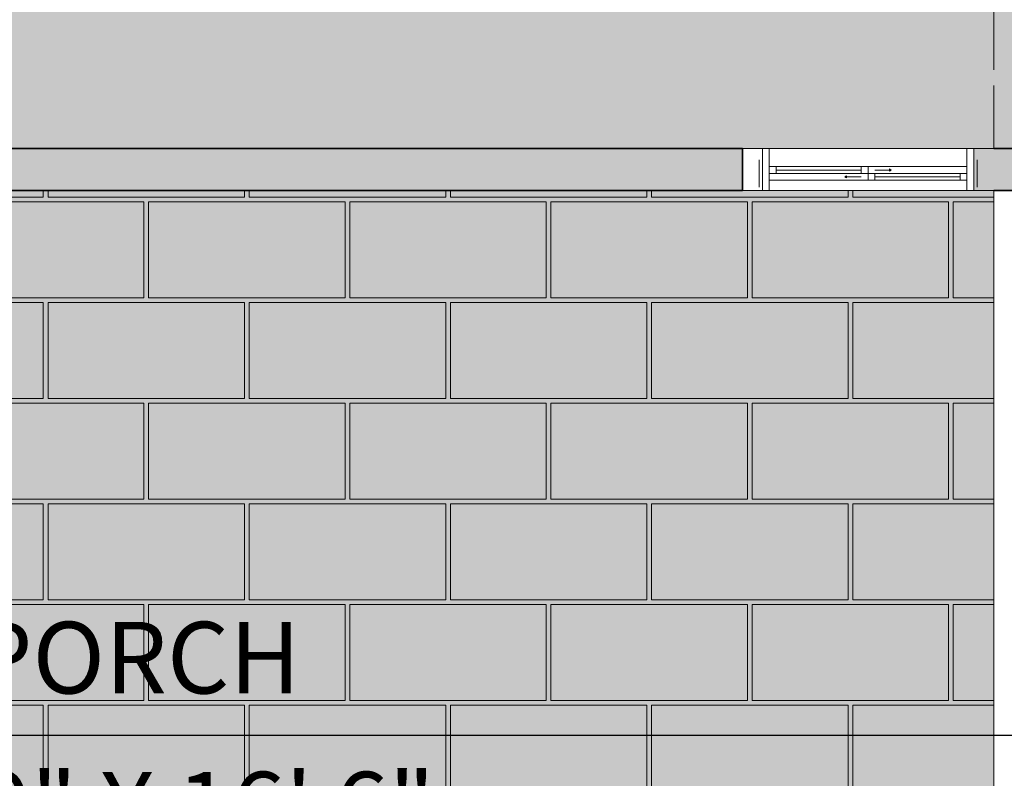
# Model space of a CAD drawing. Units: inches. Extents: x 1704 to 6393, y -157 to 1172.
# Tile 20 of 122: x 2087 to 2275, y 82 to 227. Entities that reach past the tile are written whole.
import ezdxf

# ---------------------------------------------------------------- set-up
doc = ezdxf.new("R2010")
doc.units = ezdxf.units.IN
doc.header["$MEASUREMENT"] = 0
doc.linetypes.add('ACAD_ISO02W100', pattern=[15, 12, -3])
for name, color, linetype, lineweight in [('A-ANNO-DIMS', 7, 'Continuous', 13), ('A-AREA-IDEN', 7, 'Continuous', 18), ('A-WALL-OVHD', 8, 'ACAD_ISO02W100', 13), ('A-WALL-PATT', 7, 'Continuous', 13), ('L-HRDS', 8, 'Continuous', 18), ('L-PVMT-PATT', 8, 'Continuous', 13), ('WALLS', 7, 'Continuous', 35), ('WINDOWS', 2, 'Continuous', 18)]:
    doc.layers.add(name, color=color, linetype=linetype, lineweight=lineweight)
doc.layers.add('A-FLOR-PATT', color=7, linetype='Continuous', lineweight=13, true_color=0xf2f2f2)
doc.layers.add('L-HRDS-PATT', color=9, linetype='Continuous', lineweight=13, true_color=0xc5c1ba)
doc.styles.get("Standard").update_dxf_attribs({"font": 'arial.ttf'})
doc.dimstyles.get("Standard").update_dxf_attribs({"dimtxt": 6, "dimasz": 2, "dimexe": 0.18, "dimexo": 0.0625, "dimgap": 0.09, "dimtad": 0, "dimtih": 1, "dimtoh": 1, "dimdec": 1, "dimzin": 0, "dimdsep": 46, "dimlunit": 3, "dimtxsty": 'Standard', "dimblk": 'ARCHTICK', "dimcen": 0.09, "dimadec": 0, "dimazin": 0, "dimtfac": 1, "dimtdec": 1, "dimtofl": 0, "dimtmove": 0, "dimatfit": 3, "dimfxl": 1, "dimtolj": 1, "dimtzin": 0, "dimarcsym": 0})

# ---------------------------------------------------------------- blocks, each defined once
blk = doc.blocks.new('WIN-SLIDER-48')
for p, q in [((3.83, 8), (0, 8)), ((5.13, 8), (42.87, 8)), ((44.17, 8), (48, 8)), ((3.18, 5.86), (3.18, 0.65)), ((44.82, 5.86), (44.82, 0.65)), ((6.43, 4.55), (22.7, 4.55)), ((6.43, 3.9), (22.7, 3.9)), ((24, 4.55), (42.87, 4.55)), ((25.3, 3.9), (28.1, 3.9)), ((24, 1.95), (5.13, 1.95)), ((6.43, 3.25), (22.7, 3.25)), ((22.7, 2.6), (19.9, 2.6)), ((25.3, 3.25), (41.56, 3.25)), ((25.3, 2.6), (41.56, 2.6)), ((25.3, 1.95), (41.56, 1.95)), ((3.83, 0), (0, 0)), ((5.13, 0), (42.87, 0)), ((44.17, 0), (48, 0))]:
    blk.add_line(p, q)
for points in [[(5.13, 0), (3.83, 0), (3.83, 8), (5.13, 8)], [(42.87, 0), (44.17, 0), (44.17, 8), (42.87, 8)], [(5.13, 3.25), (6.43, 3.25), (6.43, 4.55), (5.13, 4.55)], [(22.7, 3.25), (24, 3.25), (24, 4.55), (22.7, 4.55)], [(28.43, 3.9), (28.1, 4.1), (28.1, 3.71)], [(19.57, 2.6), (19.9, 2.8), (19.9, 2.41)], [(24, 1.95), (25.3, 1.95), (25.3, 3.25), (24, 3.25)], [(41.56, 1.95), (42.87, 1.95), (42.87, 3.25), (41.56, 3.25)]]:
    blk.add_lwpolyline(points, close=True)
blk = doc.blocks.new('_ArchTick')
at = {"color": 0, "linetype": 'ByBlock', "const_width": 0.15}
blk.add_lwpolyline([(-0.5, -0.5), (0.5, 0.5)], dxfattribs=at)
blk = doc.blocks.new('*D93')
at = {"layer": 'A-ANNO-DIMS', "color": 0, "lineweight": -2, "transparency": 16777216}
for p, q in [((2605.29, 895.21), (1829.7, 895.21)), ((1829.88, 895.21), (1829.88, 495.87)), ((1829.88, 90.21), (1829.88, 489.56)), ((2605.29, 90.21), (1829.7, 90.21))]:
    blk.add_line(p, q, dxfattribs=at)
at = {"layer": 'Defpoints', "color": 0, "lineweight": -3, "transparency": 16777216}
for p in [(2605.35, 895.21), (1829.88, 90.21), (2605.35, 90.21)]:
    blk.add_point(p, dxfattribs=at)
at = {"layer": 'A-ANNO-DIMS', "color": 0, "lineweight": -2, "transparency": 16777216, "xscale": 2, "yscale": 2, "zscale": 2}
for p, rotation in [((1829.88, 895.21), 90), ((1829.88, 90.21), 270)]:
    blk.add_blockref('_ArchTick', p, dxfattribs=dict(at, rotation=rotation))
at = {"layer": 'A-ANNO-DIMS', "color": 0, "transparency": 16777216, "insert": (1829.88, 492.71), "char_height": 6, "attachment_point": 5}
blk.add_mtext('\\A1;805', dxfattribs=at)

msp = doc.modelspace()

# ---------------------------------------------------------------- hatches: boundary and pattern name
at = {"layer": 'A-FLOR-PATT', "transparency": 33554528}
h = msp.add_hatch(color=256, dxfattribs=at)
h.dxf.hatch_style = 1
h.paths.add_polyline_path([(2273.349, 538.213), (2081.349, 538.213), (2081.349, 372.213), (2273.349, 372.213)])
h.paths.add_polyline_path([(2189.542, 505.951), (2184.316, 505.951), (2184.316, 505.591), (2169.442, 505.591), (2169.442, 505.951), (2164.216, 505.951, -0.4142136), (2163.814, 506.353), (2163.814, 526.093, -0.4142136), (2164.216, 526.495), (2189.542, 526.495, -0.4142136), (2189.944, 526.093), (2189.944, 506.353, -0.4142136)], flags=16)
h.paths.add_polyline_path([(2200.535, 511.491), (2200.535, 526.191), (2217.621, 526.191), (2217.621, 511.491), (2214.605, 511.491, -0.3946213), (2214.203, 511.116), (2203.952, 511.116, -0.3946213), (2203.551, 511.491)], flags=16)
h.paths.add_polyline_path([(2200.736, 511.692), (2200.736, 525.99), (2203.55, 525.99), (2203.55, 523.838, 0.1045605), (2214.605, 523.838), (2214.605, 525.99), (2217.42, 525.99), (2217.42, 511.692), (2214.605, 511.692), (2214.605, 523.838, -0.1045605), (2203.55, 523.838), (2203.55, 511.692)], flags=0)
h.paths.add_polyline_path([(2203.952, 511.317, -0.4142136), (2203.751, 511.518), (2203.751, 523.591, 0.099912), (2214.404, 523.591), (2214.404, 511.518, -0.4142136), (2214.203, 511.317)], flags=0)
h.paths.add_polyline_path([(2184.084, 516.015, -0.0686795), (2169.674, 516.015), (2169.674, 522.073), (2184.084, 522.073)], flags=0)
h.paths.add_polyline_path([(2183.325, 518.606, -0.0772766), (2170.433, 518.606), (2170.433, 521.123, -0.0235462), (2183.325, 521.123)], flags=0)
h.paths.add_polyline_path([(2135.029, 507.225, -0.1405189), (2135.191, 507.834, -0.0513838), (2135.029, 507.797)], flags=16)
h.paths.add_polyline_path([(2146.318, 498.997, -0.0311848), (2144.279, 499.202, -0.1719602), (2141.865, 499.263, -0.2234326), (2139.482, 499.263, -0.1719602), (2137.068, 499.202, -0.0311848), (2135.029, 498.997, -0.066975), (2135.029, 505.313, -0.0276914), (2136.841, 505.144), (2136.841, 506.777), (2136.576, 506.777), (2136.576, 507.371, 0.039911), (2145.741, 507.448, 0.2546956), (2146.318, 507.225), (2146.318, 507.269, 0.1305786), (2146.156, 507.834, -0.0704067), (2145.953, 507.935, -0.011584), (2145.714, 508.002, -0.2546956), (2145.137, 507.779, -0.2546956), (2145.361, 508.355, -0.0259693), (2145.107, 516.407, -0.0070422), (2144.025, 516.297, -0.1828112), (2142.939, 516.218, -0.2042746), (2142.015, 516.175, -0.1805419), (2139.348, 516.174, -0.0000184), (2139.345, 516.174, -0.2035615), (2138.425, 516.217, -0.0000237), (2138.421, 516.217, -0.1818152), (2137.34, 516.296, -0.0071635), (2136.24, 516.407, 0.007166), (2136.162, 518.63, 0.314303), (2135.854, 518.974, -0.1253469), (2135.537, 518.935, -0.2546956), (2135.76, 519.512, -0.0162662), (2135.67, 519.849, -0.296972), (2135.535, 520.8, -0.227702), (2135.464, 521.698, 0.1283977), (2132.757, 521.718), (2132.757, 525.785, -0.4142136), (2133.331, 526.359), (2148.015, 526.359, -0.4142136), (2148.589, 525.785), (2148.589, 521.718, -0.0118936), (2148.835, 521.65, -0.2546956), (2149.412, 521.873, -0.2546956), (2149.188, 521.296, -0.0417628), (2149.188, 508.355, -0.2546956), (2149.412, 507.779, -0.2546956), (2148.835, 508.002, -0.011584), (2148.596, 507.935, -0.2124435), (2147.949, 507.813, -0.2363999), (2147.423, 507.772, -0.3143526), (2147.126, 507.772, -0.2363999), (2146.6, 507.813, -0.0879275), (2146.318, 507.797), (2146.318, 507.225, -0.2546956), (2145.741, 507.448, -0.0042329), (2144.771, 507.371), (2144.771, 506.777), (2144.506, 506.777), (2144.506, 505.144, -0.0276914), (2146.318, 505.313, -0.066975)], flags=16)
h.paths.add_polyline_path([(2141.865, 505.047, 0.2234326), (2139.482, 505.047, 0.1738145), (2137.043, 505.1), (2137.043, 506.317), (2137.335, 506.317), (2137.335, 505.184, -0.1522072), (2139.482, 505.047, -0.2234326), (2141.865, 505.047, -0.1522072), (2144.011, 505.184), (2144.011, 506.317), (2144.304, 506.317), (2144.304, 505.1, 0.1738145)], flags=0)
h.paths.add_polyline_path([(2145.233, 522.986, 0.0079197), (2144.017, 523.111, 0.1826165), (2142.931, 523.19, 0.2042746), (2142.008, 523.233, 0.1806536), (2139.339, 523.233, 0.2042746), (2138.415, 523.19, 0.1826165), (2137.33, 523.111, 0.0079197), (2136.114, 522.986, 0.1967082), (2135.679, 523.212, 0.047677), (2135.755, 524.004), (2134.638, 521.852), (2134.376, 524.691, -0.2583282), (2135.029, 526.359, -0.0890464), (2135.632, 525.01, -0.1830277), (2145.715, 525.01, -0.0890464), (2146.318, 526.359, -0.2583282), (2146.971, 524.691), (2146.709, 521.852), (2145.592, 524.004, 0.047677), (2145.668, 523.212, 0.1967082)], flags=0)
h.paths.add_polyline_path([(2144.419, 519.027, -0.0368796), (2136.927, 519.027, -0.0368796)], flags=0)
h.paths.add_polyline_path([(2273.349, 629.213), (2213.349, 629.213), (2213.349, 573.213), (2213.349, 545.213), (2273.349, 545.213)])
h.paths.add_polyline_path([(2273.349, 711.213), (2207.349, 711.213), (2207.349, 709.213), (2231.349, 709.213), (2231.349, 707.213), (2207.349, 707.213), (2207.349, 631.213), (2273.349, 631.213)])
h.paths.add_polyline_path([(2273.349, 364.213), (2081.349, 364.213), (2081.349, 202.213), (2225.349, 202.213), (2229.181, 202.213), (2230.482, 202.213), (2268.215, 202.213), (2269.516, 202.213), (2273.349, 202.213)])
h.paths.add_polyline_path([(2203.551, 339.558, 0.3946213), (2203.952, 339.183), (2214.203, 339.183), (2214.203, 339.384), (2203.751, 339.384), (2203.751, 339.558)], flags=16)
h.paths.add_polyline_path([(2203.55, 351.7), (2203.55, 339.759), (2200.535, 339.759), (2200.535, 354.258), (2217.621, 354.258), (2217.621, 339.558), (2214.404, 339.558), (2214.404, 351.659, -0.101837)], flags=16)
h.paths.add_polyline_path([(2214.404, 354.057), (2214.605, 354.057), (2214.605, 354.258), (2214.404, 354.258)], flags=16)
h.paths.add_polyline_path([(2189.542, 334.018), (2184.316, 334.018), (2184.316, 333.658), (2169.442, 333.658), (2169.442, 334.018), (2164.216, 334.018, -0.4142136), (2163.814, 334.42), (2163.814, 354.161, -0.4142136), (2164.216, 354.563), (2189.542, 354.563, -0.4142136), (2189.944, 354.161), (2189.944, 334.42, -0.4142136)], flags=16)
h.paths.add_polyline_path([(2184.084, 344.083, -0.0686795), (2169.674, 344.083), (2169.674, 349.85), (2165.7, 350.14), (2188.058, 350.14), (2184.084, 349.85)], flags=0)
h.paths.add_polyline_path([(2183.325, 346.673, -0.0772766), (2170.433, 346.673), (2170.433, 349.19, -0.0235462), (2183.325, 349.19)], flags=0)
h.paths.add_polyline_path([(2134.638, 349.919), (2134.376, 352.758, -0.2583282), (2135.029, 354.426), (2133.331, 354.426, 0.4142136), (2132.757, 353.852), (2132.757, 349.785, -0.0886664)], flags=16)
h.paths.add_polyline_path([(2136.114, 351.053, -0.0079197), (2137.33, 351.178, -0.1826165), (2138.415, 351.257, -0.2042746), (2139.339, 351.3, -0.1806536), (2142.008, 351.3, -0.2042746), (2142.931, 351.257, -0.1826165), (2144.017, 351.178, -0.0079197), (2145.233, 351.053, -0.1967082), (2145.668, 351.279, -0.047677), (2145.592, 352.071, 0.1133241), (2135.755, 352.071, -0.047677), (2135.679, 351.279, -0.1967082)], flags=16)
h.paths.add_polyline_path([(2145.184, 346.697, 0.0331414), (2145.361, 336.423, 0.2546956), (2145.137, 335.846, 0.3030408), (2145.781, 336.164, 0.2903634), (2146.6, 335.88, 0.2363999), (2147.126, 335.839, -0.280712), (2147.275, 336.69, -0.280712), (2147.423, 335.839, 0.2363999), (2147.949, 335.88, 0.2903634), (2148.768, 336.164, 0.3030408), (2149.412, 335.846, 0.2546956), (2149.188, 336.423, 0.0417628), (2149.188, 349.363, 0.2546956), (2149.412, 349.94, 0.2546956), (2148.835, 349.717, 0.1405058), (2145.883, 349.765, -0.227702), (2145.812, 348.867, -0.296972), (2145.677, 347.916, -0.0162662), (2145.586, 347.579, -0.2546956), (2145.81, 347.002, -0.1253469), (2145.493, 347.041, 0.314303)], flags=16)
h.paths.add_polyline_path([(2135.029, 335.292, -0.1405189), (2135.191, 335.901, -0.1399435), (2134.747, 335.88, -0.2363999), (2134.22, 335.839, -0.3143526), (2133.924, 335.839, -0.280712), (2134.072, 336.69, -0.280712), (2134.22, 335.839, 0.2363999), (2134.747, 335.88, 0.2903634), (2135.566, 336.164, 0.3030408), (2136.209, 335.846, 0.2546956), (2135.985, 336.423, 0.0331414), (2136.162, 346.697, 0.314303), (2135.854, 347.041, -0.1253469), (2135.537, 347.002, -0.2546956), (2135.76, 347.579, -0.0162662), (2135.67, 347.916, -0.296972), (2135.535, 348.867, -0.2999866), (2135.599, 350.01, -0.0330719), (2135.76, 350.7, -0.3502076), (2135.604, 351.492), (2134.638, 349.919), (2135.604, 351.492, 0.3502076), (2135.76, 350.7, 0.0330719), (2135.599, 350.01, 0.2999866), (2135.535, 348.867, 0.296972), (2135.67, 347.916, 0.0279375), (2135.971, 347.698, 0.3576436), (2135.537, 347.002, 0.1253469), (2135.854, 347.041, -0.3555912), (2136.165, 346.637, -0.0329482), (2135.985, 336.423, -0.2546956), (2136.209, 335.846, -0.2546956), (2135.632, 336.069, -0.011584), (2135.393, 336.003, -0.1222327), (2135.029, 335.864)], flags=16)
h.paths.add_polyline_path([(2136.841, 335.42), (2136.783, 335.423), (2136.783, 334.844), (2136.841, 334.471)], flags=16)
h.paths.add_polyline_path([(2146.318, 327.064, -0.0311848), (2144.279, 327.269, -0.1719602), (2141.865, 327.33, -0.2234326), (2139.482, 327.33, -0.1719602), (2137.068, 327.269, -0.0311848), (2135.029, 327.064, -0.066975), (2135.029, 333.38, -0.0311848), (2137.068, 333.175, -0.1719602), (2139.482, 333.114, -0.2234326), (2141.865, 333.114, -0.1522072), (2144.011, 333.251), (2144.011, 334.384), (2144.304, 335.406, 0.0020345), (2144.771, 335.438), (2144.771, 334.844), (2144.506, 333.211, -0.0276914), (2146.318, 333.38, -0.066975)], flags=16)
h.paths.add_polyline_path([(2137.129, 334.384), (2137.335, 334.384), (2137.335, 333.251), (2137.129, 333.195)], flags=16)
h.paths.add_polyline_path([(2144.419, 347.094, -0.0368796), (2136.927, 347.094, -0.0368796)], flags=16)
h = msp.add_hatch(color=256, dxfattribs=at)
h.dxf.hatch_style = 1
h.paths.add_polyline_path([(2349.349, 372.213), (2277.349, 372.213), (2277.349, 364.213), (2349.349, 364.213)])
h.paths.add_polyline_path([(2277.349, 372.213), (2273.349, 372.213), (2273.349, 364.213), (2277.349, 364.213)])
h.paths.add_polyline_path([(2277.349, 364.213), (2273.349, 364.213), (2273.349, 202.213), (2277.349, 202.213)])
h.paths.add_polyline_path([(2277.349, 538.213), (2273.349, 538.213), (2273.349, 372.213), (2277.349, 372.213)])
h.paths.add_polyline_path([(2277.349, 629.213), (2273.349, 629.213), (2273.349, 545.213), (2277.349, 545.213)])
h.paths.add_polyline_path([(2277.349, 711.213), (2273.349, 711.213), (2273.349, 631.213), (2277.349, 631.213)])
h.paths.add_polyline_path([(2277.349, 631.213), (2273.349, 631.213), (2273.349, 629.213), (2277.349, 629.213)])
at = {"layer": 'A-WALL-PATT', "transparency": 33554643}
h = msp.add_hatch(color=256, dxfattribs=at)
h.dxf.hatch_style = 1
h.paths.add_polyline_path([(2167.349, 895.213), (2073.349, 895.213), (2073.349, 887.213), (2081.349, 887.213), (2167.349, 887.213)])
h.paths.add_polyline_path([(2465.349, 895.213), (2273.349, 895.213), (2273.349, 903.213), (2263.349, 903.213), (2263.349, 895.213), (2263.349, 887.213), (2325.349, 887.213), (2325.349, 863.213), (2333.349, 863.213), (2333.349, 887.213), (2465.349, 887.213)])
h.paths.add_polyline_path([(2533.349, 895.213), (2513.349, 895.213), (2513.349, 887.213), (2513.349, 861.213), (2517.349, 861.213), (2517.349, 887.213), (2533.349, 887.213)])
h.paths.add_polyline_path([(2605.349, 895.213), (2581.349, 895.213), (2581.349, 887.213), (2597.349, 887.213), (2597.349, 854.213), (2605.349, 854.213)])
h.paths.add_polyline_path([(2605.349, 752.213), (2629.349, 752.213), (2629.349, 716.213), (2605.349, 716.213), (2605.349, 712.213), (2719.349, 712.213), (2719.349, 716.213), (2631.349, 716.213), (2631.349, 754.213), (2605.349, 754.213), (2605.349, 794.213), (2597.349, 794.213), (2597.349, 787.213), (2517.349, 787.213), (2517.349, 813.213), (2513.349, 813.213), (2513.349, 783.213), (2517.349, 783.213), (2597.349, 783.213), (2597.349, 719.213), (2517.349, 719.213), (2517.349, 753.213), (2513.349, 753.213), (2513.349, 719.213), (2365.349, 719.213), (2365.349, 763.213), (2325.349, 763.213), (2325.349, 755.213), (2357.349, 755.213), (2357.349, 719.213), (2325.349, 719.213), (2325.349, 711.213), (2547.349, 711.213), (2547.349, 615.213), (2449.349, 615.213), (2449.349, 607.213), (2514.349, 607.213), (2514.349, 546.213), (2439.349, 546.213), (2425.349, 546.213), (2425.349, 607.213), (2425.349, 615.213), (2350.349, 615.213), (2350.349, 589.713), (2358.349, 589.713), (2358.349, 610.213), (2420.349, 610.213), (2420.349, 545.213), (2358.349, 545.213), (2358.349, 565.713), (2350.349, 565.713), (2350.349, 538.213), (2469.349, 538.213), (2469.349, 459.213), (2469.349, 372.213), (2423.349, 372.213), (2423.349, 364.213), (2473.349, 364.213), (2473.349, 318.213), (2477.349, 318.213), (2477.349, 364.213), (2547.349, 364.213), (2547.349, 352.213), (2549.349, 352.213), (2549.349, 364.213), (2597.349, 364.213), (2597.349, 328.213), (2549.349, 328.213), (2547.349, 328.213), (2547.349, 326.213), (2549.349, 326.213), (2597.349, 326.213), (2605.349, 326.213), (2605.349, 377.057), (2597.349, 377.057), (2597.349, 372.213), (2477.349, 372.213), (2477.349, 451.213), (2597.349, 451.213), (2605.349, 451.213), (2605.349, 459.213), (2597.349, 459.213), (2477.349, 459.213), (2477.349, 538.213), (2597.349, 538.213), (2597.349, 495.213), (2605.349, 495.213), (2605.349, 512.213), (2631.349, 512.213), (2631.349, 568.213), (2605.349, 568.213), (2605.349, 577.213), (2597.349, 577.213), (2597.349, 542.213), (2518.349, 542.213), (2518.349, 607.213), (2532.349, 607.213), (2605.349, 607.213), (2605.349, 615.213), (2597.349, 615.213), (2551.349, 615.213), (2551.349, 711.213), (2597.349, 711.213), (2597.349, 645.213), (2605.349, 645.213), (2605.349, 712.213), (2605.349, 716.213)])
h.paths.add_polyline_path([(2605.349, 566.213), (2629.349, 566.213), (2629.349, 514.213), (2605.349, 514.213)], flags=16)
h.paths.add_polyline_path([(2381.349, 372.213), (2349.349, 372.213), (2349.349, 202.213), (2337.349, 202.213), (2337.349, 194.213), (2349.349, 194.213), (2349.349, 90.213), (2349.349, 72.213), (2357.349, 72.213), (2357.349, 90.213), (2381.349, 90.213), (2381.349, 98.213), (2357.349, 98.213), (2357.349, 266.213), (2381.349, 266.213), (2381.349, 270.213), (2353.349, 270.213), (2353.349, 364.213), (2381.349, 364.213)])
h.paths.add_polyline_path([(2605.349, 302.213), (2597.349, 302.213), (2597.349, 270.213), (2477.349, 270.213), (2477.349, 294.213), (2473.349, 294.213), (2473.349, 270.213), (2423.349, 270.213), (2423.349, 266.213), (2597.349, 266.213), (2597.349, 218.213), (2605.349, 218.213)])
h.paths.add_polyline_path([(2605.349, 146.213), (2597.349, 146.213), (2597.349, 98.213), (2429.349, 98.213), (2429.349, 90.213), (2597.349, 90.213), (2597.349, 72.213), (2605.349, 72.213), (2605.349, 90.213)])
h.paths.add_polyline_path([(2225.349, 202.213), (2049.349, 202.213), (2049.349, 194.213), (2225.349, 194.213)])
h.paths.add_polyline_path([(2289.349, 202.213), (2277.349, 202.213), (2273.349, 202.213), (2269.516, 202.213), (2269.516, 194.213), (2273.349, 194.213), (2277.349, 194.213), (2289.349, 194.213)])
h.paths.add_polyline_path([(2273.349, 372.213), (2029.19, 372.213), (2029.19, 364.213), (2273.349, 364.213)])
h.paths.add_polyline_path([(2277.349, 545.213), (2213.349, 545.213), (2213.349, 573.213), (2205.349, 573.213), (2177.349, 573.213), (2177.349, 545.213), (2073.349, 545.213), (2073.349, 538.213), (2081.349, 538.213), (2277.349, 538.213)])
h.paths.add_polyline_path([(2181.349, 545.213), (2181.349, 569.213), (2205.349, 569.213), (2205.349, 545.213)], flags=16)
h.paths.add_polyline_path([(2277.349, 719.213), (2081.349, 719.213), (2073.349, 719.213), (2073.349, 711.213), (2154.575, 711.213), (2205.349, 711.213), (2205.349, 687.213), (2205.349, 629.213), (2213.349, 629.213), (2273.349, 629.213), (2273.349, 631.213), (2207.349, 631.213), (2207.349, 707.213), (2231.349, 707.213), (2231.349, 709.213), (2207.349, 709.213), (2207.349, 711.213), (2277.349, 711.213)])
at = {"layer": 'L-HRDS-PATT', "transparency": 33554646}
h = msp.add_hatch(color=256, dxfattribs=at)
h.dxf.hatch_style = 1
h.paths.add_polyline_path([(2273.349, 194.213), (2269.516, 194.213), (2268.215, 194.213), (2230.482, 194.213), (2229.181, 194.213), (2225.349, 194.213), (2049.349, 194.213), (2049.349, 202.213), (1975.349, 202.213), (1975.349, -3.787), (2273.349, -3.787)])
at = {"layer": 'L-PVMT-PATT', "transparency": 33554643}
h = msp.add_hatch(dxfattribs=at)
h.set_pattern_fill('AR-B816C', color=256, scale=2.4)
h.paths.add_polyline_path([(2273.349, 194.213), (2269.516, 194.213), (2268.215, 194.213), (2230.482, 194.213), (2229.181, 194.213), (2225.349, 194.213), (2049.349, 194.213), (2049.349, 202.213), (1975.349, 202.213), (1975.349, -3.787), (2273.349, -3.787)])

# ---------------------------------------------------------------- linework, layer by layer
at = {"layer": 'A-WALL-OVHD'}
msp.add_line((2273.349, 202.213), (2273.349, 538.213), dxfattribs=at)
at = {"layer": 'L-HRDS'}
msp.add_line((2273.349, 194.213), (2273.349, -3.787), dxfattribs=at)
at = {"layer": 'WALLS'}
for p, q in [((2225.349, 202.213), (1975.349, 202.213)), ((2225.349, 194.213), (2225.349, 202.213)), ((2277.349, 202.213), (2273.349, 202.213)), ((2225.349, 194.213), (2049.349, 194.213)), ((2277.349, 194.213), (2273.349, 194.213))]:
    msp.add_line(p, q, dxfattribs=at)

# ---------------------------------------------------------------- block references
at = {"layer": 'WINDOWS'}
msp.add_blockref('WIN-SLIDER-48', (2225.349, 194.213), dxfattribs=at)

# ---------------------------------------------------------------- texts
at = {"layer": 'A-ANNO-DIMS'}
msp.add_text('24\' 10" X 16\' 6"', height=13.6672, dxfattribs=at).set_placement((2038.807, 69.622))
at = {"layer": 'A-AREA-IDEN'}
msp.add_text('CAR PORCH', height=13.6672, dxfattribs=at).set_placement((2038.807, 98.244))

# ---------------------------------------------------------------- dimensions: what is measured, and where the dimension line sits
at = {"layer": 'A-ANNO-DIMS'}
dim = msp.add_linear_dim(base=(1829.878, 90.213), p1=(2605.349, 895.213), p2=(2605.349, 90.213), angle=90, dimstyle='Standard', override={"dimdec": 0, "dimlfac": 1, "dimrnd": 0, "dimzin": 0, "dimdsep": 46, "dimlunit": 2}, dxfattribs=at)
dim.commit()
dim.dimension.update_dxf_attribs({"geometry": '*D93', "text_midpoint": (1829.878, 492.713)})

doc.saveas('drawing.dxf')
